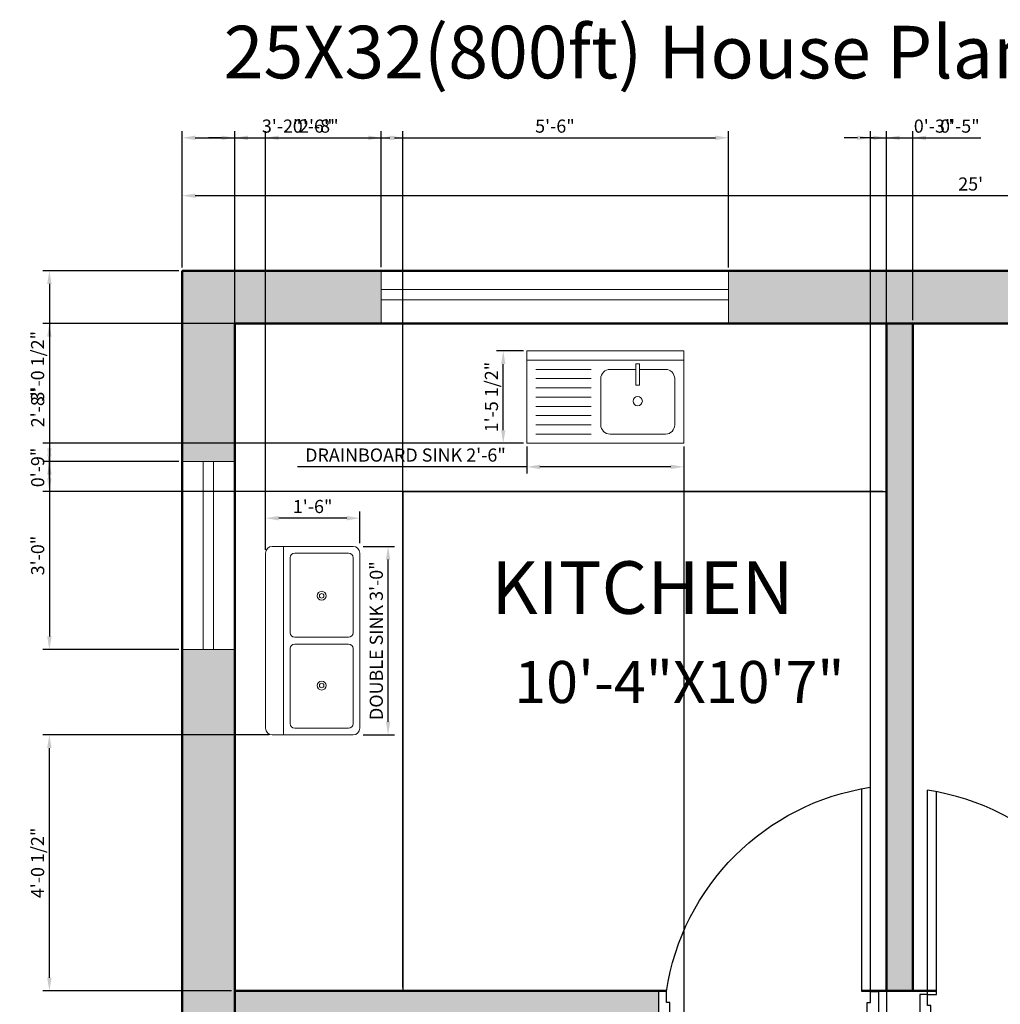
# Model space of a CAD drawing. Units: inches. Extents: x 3578 to 3951, y 1675 to 2189.
# Tile 3 of 4: x 3578 to 3765, y 2001 to 2189. Entities that reach past the tile are written whole.
import ezdxf

# ---------------------------------------------------------------- set-up
doc = ezdxf.new("R2010")
doc.units = ezdxf.units.IN
for name, color, linetype, lineweight in [('A-ANNO-DIMS', 2, 'Continuous', 18), ('A-ANNO-TEXT', 7, 'Continuous', 25), ('A-AREA-IDEN', 7, 'Continuous', 25), ('A-DOOR', 3, 'Continuous', 25), ('A-FLOR-CASE', 9, 'Continuous', 25), ('A-FLOR-FIXT', 9, 'Continuous', 18), ('A-GLAZ', 4, 'Continuous', 18), ('A-WALL', 7, 'Continuous', 50), ('A-WALL-PATT', 8, 'Continuous', 13)]:
    doc.layers.add(name, color=color, linetype=linetype, lineweight=lineweight)
doc.styles.add('ATTR', font='romans.shx', dxfattribs={"width": 0.8, "height": 1.075})
doc.styles.get("Standard").update_dxf_attribs({"font": 'arial.ttf'})
doc.dimstyles.new('ISO-25', dxfattribs={"dimtxt": 2.5, "dimasz": 2.5, "dimexe": 1.25, "dimexo": 0.625, "dimtad": 1, "dimdec": 0, "dimlunit": 4, "dimtxsty": 'Standard', "dimcen": 2.5, "dimadec": 0, "dimazin": 0, "dimtfac": 1, "dimtdec": 0, "dimtmove": 0, "dimatfit": 3, "dimfxl": 1, "dimarcsym": 0})

# ---------------------------------------------------------------- blocks, each defined once
blk = doc.blocks.new('A$C40E8097C')
for p, q in [((33.6, 192), (33.6, 1074.8)), ((72, 192), (72, 1068.3)), ((0, 192), (0, 0)), ((33.6, 192), (0, 192)), ((33.6, 144), (33.6, 192)), ((48, 144), (33.6, 144)), ((48, 48), (48, 144)), ((33.6, 0), (33.6, 48)), ((33.6, 48), (48, 48)), ((0, 0), (33.6, 0))]:
    blk.add_line(p, q)
blk.add_lwpolyline([(33.6, 192), (72, 192)])
blk.add_lwpolyline([(950, 192), (950, 0), (916.4, 0), (916.4, 48), (902, 48), (902, 144), (916.4, 144), (916.4, 192)], close=True)
blk.add_arc((-123.6, 34.8), 1051.8, 8.5964, 81.4036)
blk = doc.blocks.new('A$C3404121D')
for p, q in [((0, 0), (0, 500)), ((0, 500), (850, 500)), ((850, 500), (850, 0)), ((0, 450), (850, 450)), ((239.7, 430.7), (239.7, 425)), ((259.7, 430.7), (239.7, 430.7)), ((259.7, 430.7), (259.7, 315.4)), ((100, 400), (240, 400)), ((239.7, 425), (239.7, 315.4)), ((259.9, 400), (400, 400)), ((501.8, 400), (801.5, 400)), ((50, 100), (50, 350)), ((450, 100), (450, 350)), ((501.8, 350), (801.5, 350)), ((239.7, 315.4), (259.7, 315.4)), ((501.8, 300), (801.5, 300)), ((501.8, 250), (801.5, 250)), ((501.8, 200), (801.5, 200)), ((501.8, 150), (801.5, 150)), ((501.8, 100), (801.5, 100)), ((850, 0), (0, 0)), ((400, 50), (100, 50)), ((801.5, 50), (501.8, 50))]:
    blk.add_line(p, q)
blk.add_circle((250.1, 228.3), 25)
for centre, start, end in [((100, 350), 90, 180), ((400, 350), 0, 90), ((100, 100), 180, 270), ((400, 100), 270, 0)]:
    blk.add_arc(centre, 50, start, end)
blk = doc.blocks.new('*D7')
at = {"layer": 'A-ANNO-DIMS', "color": 0, "lineweight": -2, "transparency": 16777216}
for p, q in [((3609.18, 2141.39), (3609.18, 2156.32)), ((3909.18, 2141.39), (3909.18, 2156.32)), ((3611.68, 2155.07), (3906.68, 2155.07))]:
    blk.add_line(p, q, dxfattribs=at)
at = {"layer": 'A-ANNO-DIMS', "color": 0, "transparency": 16777216}
for points in [[(3611.68, 2155.48), (3611.68, 2154.65), (3609.18, 2155.07)], [(3906.68, 2155.48), (3906.68, 2154.65), (3909.18, 2155.07)]]:
    blk.add_solid(points, dxfattribs=at)
at = {"layer": 'Defpoints', "color": 0, "transparency": 16777216}
for p in [(3909.18, 2155.07), (3609.18, 2140.77), (3909.18, 2140.77)]:
    blk.add_point(p, dxfattribs=at)
at = {"layer": 'A-ANNO-DIMS', "color": 0, "transparency": 16777216, "insert": (3759.18, 2156.97), "char_height": 2.5, "attachment_point": 5}
blk.add_mtext("25'", dxfattribs=at)
blk = doc.blocks.new("42'' Sink Double PV")
for p, q in [((-21, -4), (21, -4)), ((-0.75, -18.5), (-0.75, -6.5)), ((0.75, -6.5), (0.75, -18.5))]:
    blk.add_line(p, q)
for points in [[(-19.5, 0), (19.5, 0)], [(-21, -19.5), (-21, -1.5)], [(21, -1.5), (21, -19.5)], [(-19.5, -18.5), (-19.5, -6.5)], [(-18.5, -5.5), (-1.75, -5.5)], [(1.75, -5.5), (18.5, -5.5)], [(19.5, -6.5), (19.5, -18.5)], [(-1.75, -19.5), (-18.5, -19.5)], [(18.5, -19.5), (1.75, -19.5)], [(19.5, -21), (-19.5, -21)]]:
    blk.add_lwpolyline(points)
for centre, radius in [((-10, -12.5), 1), ((-10, -12.5), 0.5), ((10, -12.5), 1), ((10, -12.5), 0.5)]:
    blk.add_circle(centre, radius)
for centre, radius, start, end in [((-19.5, -1.5), 1.5, 90, 180), ((19.5, -1.5), 1.5, 0, 90), ((-18.5, -6.5), 1, 90, 180), ((-1.75, -6.5), 1, 0, 90), ((1.75, -6.5), 1, 90, 180), ((18.5, -6.5), 1, 0, 90), ((-19.5, -19.5), 1.5, 180, 270), ((-18.5, -18.5), 1, 180, 270), ((-1.75, -18.5), 1, 270, 0), ((1.75, -18.5), 1, 180, 270), ((18.5, -18.5), 1, 270, 0), ((19.5, -19.5), 1.5, 270, 0)]:
    blk.add_arc(centre, radius, start, end)
at = {"style": 'ATTR', "width": 0.8, "flags": 9}
blk.add_attdef('ESTCODE', (0, 0), '', height=0.0084, dxfattribs=at)
blk = doc.blocks.new('*D19')
at = {"layer": 'A-ANNO-DIMS', "color": 0, "lineweight": -2, "transparency": 16777216}
for p, q in [((3674.75, 2107.33), (3674.75, 2102.22)), ((3704.64, 2107.33), (3704.64, 2102.22)), ((3674.75, 2103.47), (3631.1, 2103.47)), ((3702.14, 2103.47), (3677.25, 2103.47))]:
    blk.add_line(p, q, dxfattribs=at)
at = {"layer": 'A-ANNO-DIMS', "color": 0, "transparency": 16777216}
for points in [[(3677.25, 2103.89), (3677.25, 2103.05), (3674.75, 2103.47)], [(3702.14, 2103.89), (3702.14, 2103.05), (3704.64, 2103.47)]]:
    blk.add_solid(points, dxfattribs=at)
at = {"layer": 'Defpoints', "color": 0, "transparency": 16777216}
for p in [(3674.75, 2107.95), (3704.64, 2107.95), (3674.75, 2103.47)]:
    blk.add_point(p, dxfattribs=at)
at = {"layer": 'A-ANNO-DIMS', "color": 0, "transparency": 16777216, "insert": (3651.67, 2105.39), "char_height": 2.5, "attachment_point": 5}
blk.add_mtext('DRAINBOARD SINK 2\'-6"', dxfattribs=at)
blk = doc.blocks.new('*D20')
at = {"layer": 'A-ANNO-DIMS', "color": 0, "lineweight": -2, "transparency": 16777216}
for p, q in [((3674.12, 2125.54), (3669.01, 2125.54)), ((3670.26, 2110.45), (3670.26, 2123.04)), ((3674.12, 2107.95), (3669.01, 2107.95))]:
    blk.add_line(p, q, dxfattribs=at)
at = {"layer": 'A-ANNO-DIMS', "color": 0, "transparency": 16777216}
for points in [[(3669.85, 2123.04), (3670.68, 2123.04), (3670.26, 2125.54)], [(3669.85, 2110.45), (3670.68, 2110.45), (3670.26, 2107.95)]]:
    blk.add_solid(points, dxfattribs=at)
at = {"layer": 'Defpoints', "color": 0, "transparency": 16777216}
for p in [(3670.26, 2125.54), (3674.75, 2125.54), (3674.75, 2107.95)]:
    blk.add_point(p, dxfattribs=at)
at = {"layer": 'A-ANNO-DIMS', "color": 0, "transparency": 16777216, "insert": (3668.34, 2116.75), "char_height": 2.5, "attachment_point": 5, "rotation": 90}
blk.add_mtext('1\'-5 1/2"', dxfattribs=at)
blk = doc.blocks.new('*D23')
at = {"layer": 'A-ANNO-DIMS', "color": 0, "lineweight": -2, "transparency": 16777216}
for p, q in [((3643.6, 2088.32), (3649.61, 2088.32)), ((3648.36, 2054.97), (3648.36, 2085.82)), ((3643.6, 2052.47), (3649.61, 2052.47))]:
    blk.add_line(p, q, dxfattribs=at)
at = {"layer": 'A-ANNO-DIMS', "color": 0, "transparency": 16777216}
for points in [[(3647.94, 2085.82), (3648.77, 2085.82), (3648.36, 2088.32)], [(3647.94, 2054.97), (3648.77, 2054.97), (3648.36, 2052.47)]]:
    blk.add_solid(points, dxfattribs=at)
at = {"layer": 'Defpoints', "color": 0, "transparency": 16777216}
for p in [(3642.98, 2088.32), (3648.36, 2088.32), (3642.98, 2052.47)]:
    blk.add_point(p, dxfattribs=at)
at = {"layer": 'A-ANNO-DIMS', "color": 0, "transparency": 16777216, "insert": (3646.44, 2070.4), "char_height": 2.5, "attachment_point": 5, "rotation": 90}
blk.add_mtext('DOUBLE SINK 3\'-0"', dxfattribs=at)
blk = doc.blocks.new('*D24')
at = {"layer": 'A-ANNO-DIMS', "color": 0, "lineweight": -2, "transparency": 16777216}
for p, q in [((3625.05, 2088.95), (3625.05, 2094.95)), ((3642.98, 2088.95), (3642.98, 2094.95)), ((3640.48, 2093.7), (3627.55, 2093.7))]:
    blk.add_line(p, q, dxfattribs=at)
at = {"layer": 'A-ANNO-DIMS', "color": 0, "transparency": 16777216}
for points in [[(3627.55, 2094.12), (3627.55, 2093.28), (3625.05, 2093.7)], [(3640.48, 2094.12), (3640.48, 2093.28), (3642.98, 2093.7)]]:
    blk.add_solid(points, dxfattribs=at)
at = {"layer": 'Defpoints', "color": 0, "transparency": 16777216}
for p in [(3625.05, 2093.7), (3625.05, 2088.32), (3642.98, 2088.32)]:
    blk.add_point(p, dxfattribs=at)
at = {"layer": 'A-ANNO-DIMS', "color": 0, "transparency": 16777216, "insert": (3634.01, 2095.6), "char_height": 2.5, "attachment_point": 5}
blk.add_mtext('1\'-6"', dxfattribs=at)
blk = doc.blocks.new('*D25')
at = {"layer": 'A-ANNO-DIMS', "color": 0, "lineweight": -2, "transparency": 16777216}
for p, q in [((3609.18, 2141.39), (3609.18, 2167.33)), ((3611.68, 2166.08), (3644.57, 2166.08)), ((3647.07, 2141.45), (3647.07, 2167.33))]:
    blk.add_line(p, q, dxfattribs=at)
at = {"layer": 'A-ANNO-DIMS', "color": 0, "transparency": 16777216}
for points in [[(3611.68, 2166.49), (3611.68, 2165.66), (3609.18, 2166.08)], [(3644.57, 2166.49), (3644.57, 2165.66), (3647.07, 2166.08)]]:
    blk.add_solid(points, dxfattribs=at)
at = {"layer": 'Defpoints', "color": 0, "transparency": 16777216}
for p in [(3647.07, 2166.08), (3609.18, 2140.77), (3647.07, 2140.83)]:
    blk.add_point(p, dxfattribs=at)
at = {"layer": 'A-ANNO-DIMS', "color": 0, "transparency": 16777216, "insert": (3628.12, 2167.98), "char_height": 2.5, "attachment_point": 5}
blk.add_mtext('3\'-2"', dxfattribs=at)
blk = doc.blocks.new('*D26')
at = {"layer": 'A-ANNO-DIMS', "color": 0, "lineweight": -2, "transparency": 16777216}
for p, q in [((3647.07, 2141.45), (3647.07, 2167.33)), ((3649.57, 2166.08), (3710.63, 2166.08)), ((3713.13, 2141.39), (3713.13, 2167.33))]:
    blk.add_line(p, q, dxfattribs=at)
at = {"layer": 'A-ANNO-DIMS', "color": 0, "transparency": 16777216}
for points in [[(3649.57, 2166.49), (3649.57, 2165.66), (3647.07, 2166.08)], [(3710.63, 2166.49), (3710.63, 2165.66), (3713.13, 2166.08)]]:
    blk.add_solid(points, dxfattribs=at)
at = {"layer": 'Defpoints', "color": 0, "transparency": 16777216}
for p in [(3713.13, 2166.08), (3647.07, 2140.83), (3713.13, 2140.77)]:
    blk.add_point(p, dxfattribs=at)
at = {"layer": 'A-ANNO-DIMS', "color": 0, "transparency": 16777216, "insert": (3680.1, 2167.98), "char_height": 2.5, "attachment_point": 5}
blk.add_mtext('5\'-6"', dxfattribs=at)
blk = doc.blocks.new('*D27')
at = {"layer": 'A-ANNO-DIMS', "color": 0, "lineweight": -2, "transparency": 16777216}
for p, q in [((3608.55, 2140.77), (3582.68, 2140.77)), ((3583.93, 2138.27), (3583.93, 2106.98)), ((3608.55, 2104.48), (3582.68, 2104.48))]:
    blk.add_line(p, q, dxfattribs=at)
at = {"layer": 'A-ANNO-DIMS', "color": 0, "transparency": 16777216}
for points in [[(3583.51, 2138.27), (3584.35, 2138.27), (3583.93, 2140.77)], [(3583.51, 2106.98), (3584.35, 2106.98), (3583.93, 2104.48)]]:
    blk.add_solid(points, dxfattribs=at)
at = {"layer": 'Defpoints', "color": 0, "transparency": 16777216}
for p in [(3609.18, 2140.77), (3583.93, 2104.48), (3609.18, 2104.48)]:
    blk.add_point(p, dxfattribs=at)
at = {"layer": 'A-ANNO-DIMS', "color": 0, "transparency": 16777216, "insert": (3582.01, 2122.62), "char_height": 2.5, "attachment_point": 5, "rotation": 90}
blk.add_mtext('3\'-0 1/2"', dxfattribs=at)
blk = doc.blocks.new('*D28')
at = {"layer": 'A-ANNO-DIMS', "color": 0, "lineweight": -2, "transparency": 16777216}
for p, q in [((3608.55, 2104.48), (3582.68, 2104.48)), ((3583.93, 2101.98), (3583.93, 2071.21)), ((3608.55, 2068.71), (3582.68, 2068.71))]:
    blk.add_line(p, q, dxfattribs=at)
at = {"layer": 'A-ANNO-DIMS', "color": 0, "transparency": 16777216}
for points in [[(3583.51, 2101.98), (3584.35, 2101.98), (3583.93, 2104.48)], [(3583.51, 2071.21), (3584.35, 2071.21), (3583.93, 2068.71)]]:
    blk.add_solid(points, dxfattribs=at)
at = {"layer": 'Defpoints', "color": 0, "transparency": 16777216}
for p in [(3609.18, 2104.48), (3583.93, 2068.71), (3609.18, 2068.71)]:
    blk.add_point(p, dxfattribs=at)
at = {"layer": 'A-ANNO-DIMS', "color": 0, "transparency": 16777216, "insert": (3582.03, 2086.6), "char_height": 2.5, "attachment_point": 5, "rotation": 90}
blk.add_mtext('3\'-0"', dxfattribs=at)
blk = doc.blocks.new('*D46')
at = {"layer": 'A-ANNO-DIMS', "color": 0, "lineweight": -2, "transparency": 16777216}
for p, q in [((3740.68, 2166.08), (3738.18, 2166.08)), ((3743.18, 2131.39), (3743.18, 2167.33)), ((3743.18, 2166.08), (3748.18, 2166.08)), ((3748.18, 2131.39), (3748.18, 2167.33)), ((3750.68, 2166.08), (3761.08, 2166.08))]:
    blk.add_line(p, q, dxfattribs=at)
at = {"layer": 'A-ANNO-DIMS', "color": 0, "transparency": 16777216}
for points in [[(3740.68, 2166.49), (3740.68, 2165.66), (3743.18, 2166.08)], [(3750.68, 2166.49), (3750.68, 2165.66), (3748.18, 2166.08)]]:
    blk.add_solid(points, dxfattribs=at)
at = {"layer": 'Defpoints', "color": 0, "transparency": 16777216}
for p in [(3748.18, 2166.08), (3743.18, 2130.77), (3748.18, 2130.77)]:
    blk.add_point(p, dxfattribs=at)
at = {"layer": 'A-ANNO-DIMS', "color": 0, "transparency": 16777216, "insert": (3757.13, 2167.98), "char_height": 2.5, "attachment_point": 5}
blk.add_mtext('0\'-5"', dxfattribs=at)
blk = doc.blocks.new('*D47')
at = {"layer": 'A-ANNO-DIMS', "color": 0, "lineweight": -2, "transparency": 16777216}
for p, q in [((3619.18, 2004.39), (3619.18, 2167.33)), ((3621.68, 2166.08), (3648.68, 2166.08)), ((3651.18, 2004.39), (3651.18, 2167.33))]:
    blk.add_line(p, q, dxfattribs=at)
at = {"layer": 'A-ANNO-DIMS', "color": 0, "transparency": 16777216}
for points in [[(3621.68, 2166.49), (3621.68, 2165.66), (3619.18, 2166.08)], [(3648.68, 2166.49), (3648.68, 2165.66), (3651.18, 2166.08)]]:
    blk.add_solid(points, dxfattribs=at)
at = {"layer": 'Defpoints', "color": 0, "transparency": 16777216}
for p in [(3651.18, 2166.08), (3619.18, 2003.77), (3651.18, 2003.77)]:
    blk.add_point(p, dxfattribs=at)
at = {"layer": 'A-ANNO-DIMS', "color": 0, "transparency": 16777216, "insert": (3635.18, 2167.98), "char_height": 2.5, "attachment_point": 5}
blk.add_mtext('2\'-8"', dxfattribs=at)
blk = doc.blocks.new('*D48')
at = {"layer": 'A-ANNO-DIMS', "color": 0, "lineweight": -2, "transparency": 16777216}
for p, q in [((3742.55, 2130.77), (3582.68, 2130.77)), ((3583.93, 2128.27), (3583.93, 2101.27)), ((3742.55, 2098.77), (3582.68, 2098.77))]:
    blk.add_line(p, q, dxfattribs=at)
at = {"layer": 'A-ANNO-DIMS', "color": 0, "transparency": 16777216}
for points in [[(3583.51, 2128.27), (3584.35, 2128.27), (3583.93, 2130.77)], [(3583.51, 2101.27), (3584.35, 2101.27), (3583.93, 2098.77)]]:
    blk.add_solid(points, dxfattribs=at)
at = {"layer": 'Defpoints', "color": 0, "transparency": 16777216}
for p in [(3743.18, 2130.77), (3583.93, 2098.77), (3743.18, 2098.77)]:
    blk.add_point(p, dxfattribs=at)
at = {"layer": 'A-ANNO-DIMS', "color": 0, "transparency": 16777216, "insert": (3582.03, 2114.77), "char_height": 2.5, "attachment_point": 5, "rotation": 90}
blk.add_mtext('2\'-8"', dxfattribs=at)
blk = doc.blocks.new('*D52')
at = {"layer": 'A-ANNO-DIMS', "color": 0, "lineweight": -2, "transparency": 16777216}
for p, q in [((3616.68, 2166.08), (3614.18, 2166.08)), ((3619.18, 2131.39), (3619.18, 2167.33)), ((3619.18, 2166.08), (3625.05, 2166.08)), ((3625.05, 2087.67), (3625.05, 2167.33)), ((3627.55, 2166.08), (3637.95, 2166.08))]:
    blk.add_line(p, q, dxfattribs=at)
at = {"layer": 'A-ANNO-DIMS', "color": 0, "transparency": 16777216}
for points in [[(3616.68, 2166.49), (3616.68, 2165.66), (3619.18, 2166.08)], [(3627.55, 2166.49), (3627.55, 2165.66), (3625.05, 2166.08)]]:
    blk.add_solid(points, dxfattribs=at)
at = {"layer": 'Defpoints', "color": 0, "transparency": 16777216}
for p in [(3625.05, 2166.08), (3619.18, 2130.77), (3625.05, 2087.04)]:
    blk.add_point(p, dxfattribs=at)
at = {"layer": 'A-ANNO-DIMS', "color": 0, "transparency": 16777216, "insert": (3634, 2167.98), "char_height": 2.5, "attachment_point": 5}
blk.add_mtext('0\'-6"', dxfattribs=at)
blk = doc.blocks.new('*D53')
at = {"layer": 'A-ANNO-DIMS', "color": 0, "lineweight": -2, "transparency": 16777216}
for p, q in [((3625.71, 2052.47), (3582.68, 2052.47)), ((3583.93, 2006.27), (3583.93, 2049.97)), ((3618.55, 2003.77), (3582.68, 2003.77))]:
    blk.add_line(p, q, dxfattribs=at)
at = {"layer": 'A-ANNO-DIMS', "color": 0, "transparency": 16777216}
for points in [[(3583.51, 2049.97), (3584.35, 2049.97), (3583.93, 2052.47)], [(3583.51, 2006.27), (3584.35, 2006.27), (3583.93, 2003.77)]]:
    blk.add_solid(points, dxfattribs=at)
at = {"layer": 'Defpoints', "color": 0, "transparency": 16777216}
for p in [(3583.93, 2052.47), (3626.33, 2052.47), (3619.18, 2003.77)]:
    blk.add_point(p, dxfattribs=at)
at = {"layer": 'A-ANNO-DIMS', "color": 0, "transparency": 16777216, "insert": (3582.01, 2028.12), "char_height": 2.5, "attachment_point": 5, "rotation": 90}
blk.add_mtext('4\'-0 1/2"', dxfattribs=at)
blk = doc.blocks.new('*D54')
at = {"layer": 'A-ANNO-DIMS', "color": 0, "lineweight": -2, "transparency": 16777216}
for p, q in [((3704.64, 2107.33), (3704.64, 1696.88)), ((3743.18, 2098.14), (3743.18, 1696.88)), ((3740.68, 1698.13), (3707.14, 1698.13))]:
    blk.add_line(p, q, dxfattribs=at)
at = {"layer": 'A-ANNO-DIMS', "color": 0, "transparency": 16777216}
for points in [[(3707.14, 1698.55), (3707.14, 1697.71), (3704.64, 1698.13)], [(3740.68, 1698.55), (3740.68, 1697.71), (3743.18, 1698.13)]]:
    blk.add_solid(points, dxfattribs=at)
at = {"layer": 'Defpoints', "color": 0, "transparency": 16777216}
for p in [(3704.64, 2107.95), (3743.18, 2098.77), (3704.64, 1698.13)]:
    blk.add_point(p, dxfattribs=at)
at = {"layer": 'A-ANNO-DIMS', "color": 0, "transparency": 16777216, "insert": (3723.91, 1700.05), "char_height": 2.5, "attachment_point": 5}
blk.add_mtext('3\'-2 1/2"', dxfattribs=at)
blk = doc.blocks.new('*D55')
at = {"layer": 'A-ANNO-DIMS', "color": 0, "lineweight": -2, "transparency": 16777216}
for p, q in [((3674.12, 2107.95), (3582.68, 2107.95)), ((3583.93, 2101.27), (3583.93, 2105.45)), ((3650.55, 2098.77), (3582.68, 2098.77))]:
    blk.add_line(p, q, dxfattribs=at)
at = {"layer": 'A-ANNO-DIMS', "color": 0, "transparency": 16777216}
for points in [[(3583.51, 2105.45), (3584.35, 2105.45), (3583.93, 2107.95)], [(3583.51, 2101.27), (3584.35, 2101.27), (3583.93, 2098.77)]]:
    blk.add_solid(points, dxfattribs=at)
at = {"layer": 'Defpoints', "color": 0, "transparency": 16777216}
for p in [(3583.93, 2107.95), (3674.75, 2107.95), (3651.18, 2098.77)]:
    blk.add_point(p, dxfattribs=at)
at = {"layer": 'A-ANNO-DIMS', "color": 0, "transparency": 16777216, "insert": (3582.03, 2103.36), "char_height": 2.5, "attachment_point": 5, "rotation": 90}
blk.add_mtext('0\'-9"', dxfattribs=at)
blk = doc.blocks.new('*D58')
at = {"layer": 'A-ANNO-DIMS', "color": 0, "lineweight": -2, "transparency": 16777216}
for p, q in [((3737.64, 2166.08), (3735.14, 2166.08)), ((3740.14, 2004.28), (3740.14, 2167.33)), ((3740.14, 2166.08), (3743.18, 2166.08)), ((3743.18, 2004.39), (3743.18, 2167.33)), ((3745.68, 2166.08), (3756.08, 2166.08))]:
    blk.add_line(p, q, dxfattribs=at)
at = {"layer": 'A-ANNO-DIMS', "color": 0, "transparency": 16777216}
for points in [[(3737.64, 2166.49), (3737.64, 2165.66), (3740.14, 2166.08)], [(3745.68, 2166.49), (3745.68, 2165.66), (3743.18, 2166.08)]]:
    blk.add_solid(points, dxfattribs=at)
at = {"layer": 'Defpoints', "color": 0, "transparency": 16777216}
for p in [(3743.18, 2166.08), (3740.14, 2003.66), (3743.18, 2003.77)]:
    blk.add_point(p, dxfattribs=at)
at = {"layer": 'A-ANNO-DIMS', "color": 0, "transparency": 16777216, "insert": (3752.13, 2167.98), "char_height": 2.5, "attachment_point": 5}
blk.add_mtext('0\'-3"', dxfattribs=at)

msp = doc.modelspace()

# ---------------------------------------------------------------- hatches: boundary and pattern name
at = {"layer": 'A-WALL-PATT'}
h = msp.add_hatch(color=256, dxfattribs=at)
h.dxf.hatch_style = 1
h.paths.add_polyline_path([(3619.18, 1950.71), (3609.18, 1950.71), (3609.18, 1756.77), (3648.78, 1756.77), (3648.78, 1766.77), (3619.18, 1766.77)])
h.paths.add_polyline_path([(3619.18, 2068.71), (3609.18, 2068.71), (3609.18, 1975.57), (3619.18, 1975.57), (3619.18, 1998.77)])
h.paths.add_polyline_path([(3619.18, 2130.77), (3647.07, 2130.77), (3647.07, 2140.77), (3609.18, 2140.77), (3609.18, 2104.48), (3619.18, 2104.48)])
h.paths.add_polyline_path([(3909.18, 2140.77), (3713.13, 2140.77), (3713.13, 2130.77), (3899.18, 2130.77), (3899.18, 2110.42), (3909.18, 2110.42)])
h.paths.add_polyline_path([(3909.18, 2050.5), (3899.18, 2050.5), (3899.18, 1980.99), (3909.18, 1980.99)])
h.paths.add_polyline_path([(3909.18, 1881.86), (3899.18, 1881.86), (3899.18, 1941.89), (3890.7, 1942.45), (3889.21, 1942.68, -0.02009), (3881.89, 1944.66, -0.072677), (3876.18, 1946.94, -0.17277), (3874.16, 1950.75, -0.17277), (3875.79, 1954.64, -0.055418), (3880.27, 1956.72, -0.024581), (3889.21, 1959.22), (3890.7, 1959.45), (3899.18, 1960.01), (3899.18, 1952.98), (3909.18, 1952.98)])
h.paths.add_polyline_path([(3891.56, 1958.83, 0.100666), (3890.28, 1958.86, 0.024932), (3881.25, 1956.42, 0.064314), (3876.22, 1954.24, 0.17277), (3874.74, 1950.82, 0.17277), (3876.47, 1947.45, 0.072922), (3882.04, 1945.22, 0.022708), (3890.28, 1943.04, 0.100666), (3891.56, 1943.07, 0.125847)], flags=16)
h.paths.add_polyline_path([(3898.92, 1942.47, 0.324885), (3899.15, 1942.79), (3899.15, 1959.11, 0.551642), (3898.67, 1959.41), (3899.15, 1959.45), (3899.15, 1942.45)], flags=16)
h.paths.add_polyline_path([(3890.7, 1948.47, -1), (3891.63, 1948.47, -1)], flags=0)
h.paths.add_polyline_path([(3884.71, 1945.94, -0.104302), (3877.06, 1948.46, -0.17277), (3875.9, 1950.94, -0.17277), (3877.06, 1953.43, -0.104302), (3884.71, 1955.94, -0.414214), (3889.71, 1950.94, -0.414214)], flags=0)
h.paths.add_polyline_path([(3887.07, 1948.79), (3885.02, 1950.11, -0.031181), (3884.52, 1950.35, -0.229141), (3884.09, 1950.94, -0.229141), (3884.52, 1951.54, -0.109107), (3886.35, 1952.09, -0.199237), (3886.5, 1952.04, -0.461153), (3886.5, 1949.84), (3887.38, 1949.28)], flags=0)
h.paths.add_polyline_path([(3890.7, 1953.43, -1), (3891.63, 1953.43, -1)], flags=0)
h.paths.add_polyline_path([(3909.18, 1843.84), (3899.18, 1843.84), (3899.18, 1766.77), (3844.49, 1766.77), (3844.49, 1756.77), (3909.18, 1756.77)])
h = msp.add_hatch(color=256, dxfattribs=at)
h.dxf.hatch_style = 1
h.paths.add_polyline_path([(3899.18, 2003.77), (3789.71, 2003.77, -0.003692), (3789.81, 2003.09), (3791.29, 2003.09), (3791.29, 1998.77), (3899.18, 1998.77)])
h.paths.add_polyline_path([(3748.18, 2130.77), (3743.18, 2130.77), (3743.18, 2003.77), (3748.18, 2003.77)])
h.paths.add_polyline_path([(3899.18, 1920.77), (3864.53, 1920.77), (3864.53, 1915.77), (3899.18, 1915.77)], flags=0)
h.paths.add_polyline_path([(3748.18, 1872.53), (3743.18, 1872.53), (3743.18, 1766.77), (3748.18, 1766.77)], flags=0)
h.paths.add_polyline_path([(3807.15, 1834.35), (3847.1, 1834.35), (3847.1, 1854.95), (3807.15, 1854.95)], flags=8)
h.paths.add_polyline_path([(3791.36, 1816.7), (3859.75, 1816.7), (3859.75, 1833.18), (3791.36, 1833.18)], flags=8)
h.paths.add_polyline_path([(3771.09, 1986.79), (3779.29, 1986.79), (3779.29, 1991.94), (3771.09, 1991.94)], flags=8)
h.paths.add_polyline_path([(3782.02, 1935.64), (3790.22, 1935.64), (3790.22, 1940.79), (3782.02, 1940.79)], flags=8)
h = msp.add_hatch(color=256, dxfattribs=at)
h.dxf.hatch_style = 1
h.paths.add_polyline_path([(3748.18, 1872.53), (3743.18, 1872.53), (3743.18, 1766.77), (3748.18, 1766.77)], flags=0)
h.paths.add_polyline_path([(3815.97, 1920.2), (3822.72, 1920.2), (3822.72, 1920.6), (3824.18, 1920.6), (3824.18, 1998.77), (3791.29, 1998.77), (3791.29, 1994.64), (3789.81, 1994.64), (3789.81, 1996.75), (3789.18, 1996.75), (3789.18, 1998.77), (3751.6, 1998.77), (3751.6, 1996.75), (3750.96, 1996.75), (3750.96, 1994.64), (3749.49, 1994.64), (3749.49, 1998.77), (3741.62, 1998.77), (3741.62, 1995.21), (3740.14, 1995.21), (3740.14, 1997.32), (3739.51, 1997.32), (3739.51, 1998.77), (3726.18, 1998.77), (3726.18, 1920.73), (3726.07, 1920.73), (3619.18, 1920.77), (3619.18, 1915.77), (3743.18, 1915.77), (3743.18, 1914.33), (3751.33, 1914.33), (3751.33, 1912.86), (3749.22, 1912.86), (3749.22, 1912.22), (3745, 1912.22), (3745, 1912.86), (3742.88, 1912.86), (3742.88, 1911.17), (3704.32, 1911.17, 0.31859), (3742.88, 1874.01), (3745, 1874.01), (3745, 1874.64), (3749.22, 1874.64), (3749.22, 1874.01), (3751.33, 1874.01), (3751.33, 1872.53), (3748.18, 1872.53), (3748.18, 1766.77), (3751.55, 1766.77), (3751.55, 1767.57), (3753.03, 1767.57), (3753.03, 1806.42, -0.328818), (3791.88, 1767.57), (3793.35, 1767.57), (3793.35, 1766.77), (3899.18, 1766.77), (3899.18, 1915.77), (3864.53, 1915.77), (3864.53, 1912.15), (3863.05, 1912.15), (3863.05, 1914.26), (3862.42, 1914.26), (3862.42, 1915.77), (3824.84, 1915.77), (3824.84, 1914.26), (3824.2, 1914.26), (3824.2, 1912.15), (3822.72, 1912.15), (3822.72, 1915.77), (3815.97, 1915.77)], flags=17)
h.paths.add_polyline_path([(3815.97, 1920.2), (3822.72, 1920.2), (3822.72, 1920.6), (3824.18, 1920.6), (3824.18, 1998.77), (3791.29, 1998.77), (3791.29, 1994.64), (3789.81, 1994.64), (3789.81, 1996.75), (3789.18, 1996.75), (3789.18, 1998.77), (3751.6, 1998.77), (3751.6, 1996.75), (3750.96, 1996.75), (3750.96, 1994.64), (3749.49, 1994.64), (3749.49, 1998.77), (3741.62, 1998.77), (3741.62, 1995.21), (3740.14, 1995.21), (3740.14, 1997.32), (3739.51, 1997.32), (3739.51, 1998.77), (3726.18, 1998.77), (3726.18, 1920.73), (3619.18, 1920.77), (3619.18, 1915.77), (3743.18, 1915.77), (3743.18, 1914.33), (3751.33, 1914.33), (3751.33, 1912.86), (3749.22, 1912.86), (3749.22, 1912.22), (3745, 1912.22), (3745, 1912.86), (3742.88, 1912.86), (3742.88, 1911.17), (3704.32, 1911.17, 0.31859), (3742.88, 1874.01), (3745, 1874.01), (3745, 1874.64), (3749.22, 1874.64), (3749.22, 1874.01), (3751.33, 1874.01), (3751.33, 1872.53), (3748.18, 1872.53), (3748.18, 1766.77), (3751.55, 1766.77), (3751.55, 1767.57), (3753.03, 1767.57), (3753.03, 1806.42, -0.328818), (3791.88, 1767.57), (3793.35, 1767.57), (3793.35, 1766.77), (3899.18, 1766.77), (3899.18, 1915.77), (3864.53, 1915.77), (3864.53, 1912.15), (3863.05, 1912.15), (3863.05, 1914.26), (3862.42, 1914.26), (3862.42, 1915.77), (3824.84, 1915.77), (3824.84, 1914.26), (3824.2, 1914.26), (3824.2, 1912.15), (3822.72, 1912.15), (3822.72, 1915.77), (3815.97, 1915.77)], flags=17)
h.paths.add_polyline_path([(3699.81, 2003.77), (3619.18, 2003.77), (3619.18, 1998.77), (3699.81, 1998.77)])
h.paths.add_polyline_path([(3807.15, 1834.35), (3847.1, 1834.35), (3847.1, 1854.95), (3807.15, 1854.95)], flags=8)
h.paths.add_polyline_path([(3791.36, 1816.7), (3859.75, 1816.7), (3859.75, 1833.18), (3791.36, 1833.18)], flags=8)

# ---------------------------------------------------------------- linework, layer by layer
at = {"layer": 'A-FLOR-CASE'}
for q in [(3651.18, 2003.77), (3743.18, 2098.77)]:
    msp.add_line((3651.18, 2098.77), q, dxfattribs=at)
at = {"layer": 'A-GLAZ'}
for p, q in [((3647.07, 2140.83), (3647.07, 2130.77)), ((3713.13, 2140.77), (3713.13, 2130.77)), ((3647.07, 2137.23), (3713.13, 2137.23)), ((3647.07, 2135.23), (3713.13, 2135.23)), ((3619.18, 2104.48), (3609.18, 2104.48)), ((3613.18, 2068.71), (3613.18, 2104.48)), ((3615.18, 2068.71), (3615.18, 2104.48)), ((3619.18, 2068.71), (3609.18, 2068.71))]:
    msp.add_line(p, q, dxfattribs=at)
at = {"layer": 'A-WALL'}
for p, q in [((3609.18, 2140.77), (3909.18, 2140.77)), ((3609.18, 1756.77), (3609.18, 2140.77)), ((3619.18, 2130.77), (3899.18, 2130.77)), ((3619.18, 1766.77), (3619.18, 2130.77)), ((3619.18, 2130.77), (3619.18, 2003.77)), ((3743.18, 2003.77), (3743.18, 2130.77)), ((3748.18, 2003.77), (3748.18, 2130.77)), ((3619.18, 2003.77), (3701.31, 2003.77)), ((3738.45, 2003.77), (3752.65, 2003.77))]:
    msp.add_line(p, q, dxfattribs=at)

# ---------------------------------------------------------------- block references
at = {"layer": 'A-DOOR', "yscale": 0.044006868052547, "zscale": 0.044006868052547}
for p, xscale in [((3741.62, 1995.21), -0.044006868052547), ((3749.49, 1994.64), 0.044006868052547)]:
    msp.add_blockref('A$C40E8097C', p, dxfattribs=dict(at, xscale=xscale))
at = {"layer": 'A-FLOR-FIXT', "xscale": -0.0351686352301006, "yscale": 0.0351686352301006, "zscale": 0.0351686352301006}
msp.add_blockref('A$C3404121D', (3704.64, 2107.95), dxfattribs=at)
at = {"layer": 'A-FLOR-FIXT', "xscale": 0.8535817510614183, "yscale": 0.8535817510614183, "zscale": 0.8535817510614183, "rotation": 90}
msp.add_blockref("42'' Sink Double PV", (3625.05, 2070.4), dxfattribs=at)

# ---------------------------------------------------------------- texts
at = {"layer": 'A-ANNO-TEXT', "insert": (3617.08, 2187.39), "char_height": 10, "attachment_point": 1}
msp.add_mtext('25X32(800ft) House Plan-North Face-Fp1064', dxfattribs=at)
at = {"layer": 'A-AREA-IDEN', "attachment_point": 1}
for s, insert, char_height in [('KITCHEN', (3667.99, 2085.5), 10), ('10\'-4"X10\'7"', (3672.37, 2066.53), 8)]:
    msp.add_mtext(s, dxfattribs=dict(at, insert=insert, char_height=char_height))

# ---------------------------------------------------------------- dimensions: what is measured, and where the dimension line sits
at = {"layer": 'A-ANNO-DIMS'}
for base, p1, p2, override, picture, middle in [((3647.07, 2166.08), (3609.18, 2140.77), (3647.07, 2140.83), {"dimdec": 1, "dimlfac": 1, "dimrnd": 0, "dimzin": 1, "dimdsep": 46, "dimlunit": 4, "dimfrac": 2}, '*D25', (3628.12, 2167.98)), ((3625.05, 2166.08), (3619.18, 2130.77), (3625.05, 2087.04), {"dimdec": 1, "dimlfac": 1, "dimrnd": 0, "dimzin": 1, "dimdsep": 46, "dimlunit": 4, "dimfrac": 2}, '*D52', (3634, 2167.98)), ((3651.18, 2166.08), (3619.18, 2003.77), (3651.18, 2003.77), {"dimdec": 1, "dimlfac": 1, "dimrnd": 0, "dimzin": 1, "dimdsep": 46, "dimlunit": 4, "dimfrac": 2}, '*D47', (3635.18, 2167.98)), ((3713.13, 2166.08), (3647.07, 2140.83), (3713.13, 2140.77), {"dimdec": 1, "dimlfac": 1, "dimrnd": 0, "dimzin": 1, "dimdsep": 46, "dimlunit": 4, "dimfrac": 2}, '*D26', (3680.1, 2167.98)), ((3743.18, 2166.08), (3740.14, 2003.66), (3743.18, 2003.77), {"dimdec": 1, "dimlfac": 1, "dimrnd": 0, "dimzin": 1, "dimdsep": 46, "dimlunit": 4, "dimfrac": 2}, '*D58', (3752.13, 2167.98)), ((3748.18, 2166.08), (3743.18, 2130.77), (3748.18, 2130.77), {"dimdec": 1, "dimlfac": 1, "dimrnd": 0, "dimzin": 1, "dimdsep": 46, "dimlunit": 4, "dimfrac": 2}, '*D46', (3757.13, 2167.98)), ((3909.18, 2155.07), (3609.18, 2140.77), (3909.18, 2140.77), {"dimclrd": 0, "dimclre": 0, "dimclrt": 0}, '*D7', (3759.18, 2156.97)), ((3704.64, 1698.13), (3743.18, 2098.77), (3704.64, 2107.95), {"dimdec": 1, "dimlfac": 1, "dimrnd": 0, "dimzin": 1, "dimdsep": 46, "dimlunit": 4, "dimfrac": 2}, '*D54', (3723.91, 1700.05))]:
    dim = msp.add_linear_dim(base=base, p1=p1, p2=p2, dimstyle='ISO-25', override=override, dxfattribs=at)
    dim.commit()
    dim.dimension.update_dxf_attribs({"geometry": picture, "text_midpoint": middle})
for base, p1, p2, angle, picture, middle in [((3583.93, 2104.48), (3609.18, 2140.77), (3609.18, 2104.48), 90, '*D27', (3582.01, 2122.62)), ((3583.93, 2098.77), (3743.18, 2130.77), (3743.18, 2098.77), 90, '*D48', (3582.03, 2114.77)), ((3670.26, 2125.54), (3674.75, 2107.95), (3674.75, 2125.54), 90, '*D20', (3668.34, 2116.75)), ((3583.93, 2107.95), (3651.18, 2098.77), (3674.75, 2107.95), 90, '*D55', (3582.03, 2103.36)), ((3583.93, 2068.71), (3609.18, 2104.48), (3609.18, 2068.71), 90, '*D28', (3582.03, 2086.6)), ((3625.05, 2093.7), (3642.98, 2088.32), (3625.05, 2088.32), 180, '*D24', (3634.01, 2095.6)), ((3583.93, 2052.47), (3619.18, 2003.77), (3626.33, 2052.47), 90, '*D53', (3582.01, 2028.12))]:
    dim = msp.add_linear_dim(base=base, p1=p1, p2=p2, angle=angle, dimstyle='ISO-25', override={"dimdec": 1, "dimlfac": 1, "dimrnd": 0, "dimzin": 1, "dimdsep": 46, "dimlunit": 4, "dimfrac": 2}, dxfattribs=at)
    dim.commit()
    dim.dimension.update_dxf_attribs({"geometry": picture, "text_midpoint": middle})
for base, p1, p2, angle, text, picture, middle in [((3674.75, 2103.47), (3704.64, 2107.95), (3674.75, 2107.95), 180, 'DRAINBOARD SINK <>', '*D19', (3651.67, 2105.39)), ((3648.3562, 2088.3234), (3642.9787, 2052.473), (3642.9787, 2088.3234), 90, 'DOUBLE SINK <>', '*D23', (3646.4369, 2070.3982))]:
    dim = msp.add_linear_dim(base=base, p1=p1, p2=p2, angle=angle, text=text, dimstyle='ISO-25', override={"dimdec": 1, "dimlfac": 1, "dimrnd": 0, "dimzin": 1, "dimdsep": 46, "dimlunit": 4, "dimfrac": 2}, dxfattribs=at)
    dim.commit()
    dim.dimension.update_dxf_attribs({"geometry": picture, "text_midpoint": middle})

doc.saveas('drawing.dxf')
